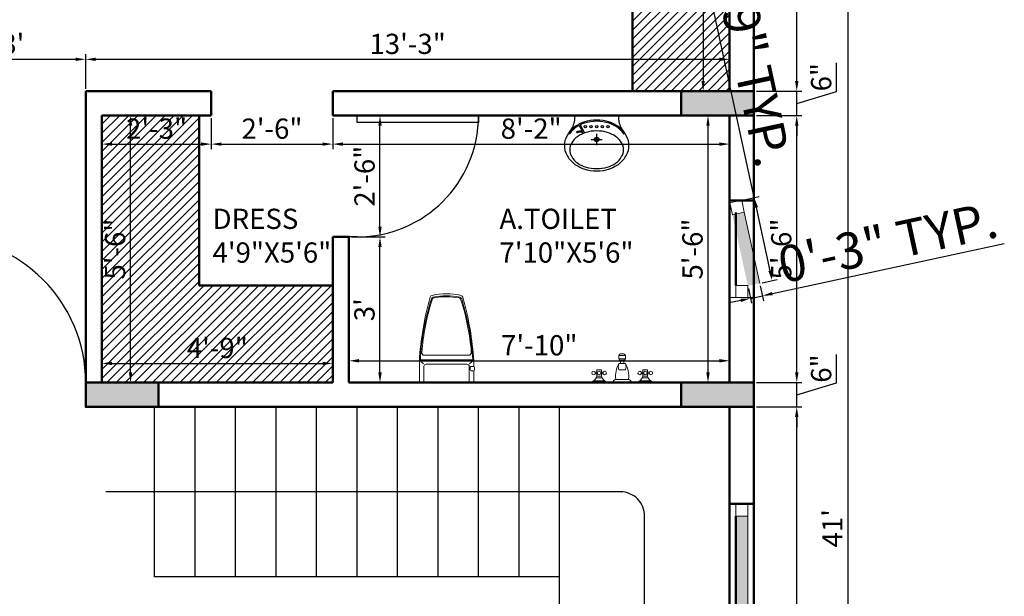
# Model space of a CAD drawing. Units: inches. Extents: x 3064 to 19385, y 846 to 15425.
# Tile 102 of 108: x 7687 to 7930, y 1134 to 1276. Entities that reach past the tile are written whole.
import ezdxf

# ---------------------------------------------------------------- set-up
doc = ezdxf.new("R2010")
doc.units = ezdxf.units.IN
for name, color, linetype, lineweight in [('A-ANNO-DIMS', 2, 'Continuous', 18), ('A-AREA-IDEN', 3, 'Continuous', 18), ('A-COLS', 1, 'Continuous', 35), ('A-DOOR', 3, 'Continuous', 25), ('A-FLOR-FIXT', 9, 'Continuous', 18), ('A-FLOR-STRS', 2, 'Continuous', 25), ('A-FURN-PATT', 252, 'Continuous', 13), ('A-GLAZ', 4, 'Continuous', 18), ('A-WALL', 7, 'Continuous', 50)]:
    doc.layers.add(name, color=color, linetype=linetype, lineweight=lineweight)
doc.layers.add('THIET-BI', color=21, linetype='Continuous')
doc.styles.get("Standard").update_dxf_attribs({"font": 'arial.ttf'})
doc.dimstyles.new('ISO-25', dxfattribs={"dimtxt": 9, "dimasz": 2.5, "dimexe": 1.25, "dimexo": 0.625, "dimtad": 1, "dimdec": 1, "dimlunit": 3, "dimtxsty": 'Standard', "dimcen": 2.5, "dimadec": 0, "dimazin": 0, "dimtfac": 1, "dimtdec": 1, "dimtmove": 0, "dimatfit": 3, "dimfxl": 1, "dimarcsym": 0})
pattern_1 = [(45, (3183.7531, 0), (-1.122532, 1.122532), [])]

# ---------------------------------------------------------------- blocks, each defined once
blk = doc.blocks.new('*U3')
for p, q in [((0, 0), (0, -6)), ((36, 0), (36, -6))]:
    blk.add_line(p, q)
blk.add_lwpolyline([(0, 0), (0, 36), (1.75, 36), (1.75, 0)], close=True)
blk.add_arc((0, 0), 36, 0, 90)
blk = doc.blocks.new('*U4')
for p, q in [((0, 0), (0, -6)), ((30, 0), (30, -6))]:
    blk.add_line(p, q)
blk.add_lwpolyline([(0, 0), (0, 30), (1.75, 30), (1.75, 0)], close=True)
blk.add_arc((0, 0), 30, 0, 90)
blk = doc.blocks.new('*D329')
at = {"layer": 'A-ANNO-DIMS', "color": 0, "lineweight": -2, "transparency": 16777216}
for p, q in [((7868.87, 1180.34), (7880.08, 1180.34)), ((7878.83, 984.84), (7878.83, 1177.84)), ((7862.87, 982.34), (7880.08, 982.34))]:
    blk.add_line(p, q, dxfattribs=at)
at = {"layer": 'A-ANNO-DIMS', "color": 0, "transparency": 16777216}
for points in [[(7878.41, 1177.84), (7879.25, 1177.84), (7878.83, 1180.34)], [(7878.41, 984.84), (7879.25, 984.84), (7878.83, 982.34)]]:
    blk.add_solid(points, dxfattribs=at)
at = {"layer": 'Defpoints', "color": 0, "transparency": 16777216}
for p in [(7868.25, 1180.34), (7878.83, 1180.34), (7862.25, 982.34)]:
    blk.add_point(p, dxfattribs=at)
at = {"layer": 'A-ANNO-DIMS', "color": 0, "transparency": 16777216, "insert": (7875.65, 1081.34), "char_height": 5, "attachment_point": 5, "rotation": 90}
blk.add_mtext('16\'-6"', dxfattribs=at)
blk = doc.blocks.new('*D330')
at = {"layer": 'A-ANNO-DIMS', "color": 0, "lineweight": -2, "transparency": 16777216}
for p, q in [((7878.83, 1188.84), (7878.83, 1191.34)), ((7888.67, 1186.29), (7888.67, 1193.32)), ((7868.87, 1186.34), (7880.08, 1186.34)), ((7878.83, 1180.34), (7878.83, 1186.34)), ((7878.83, 1180.34), (7878.83, 1186.34)), ((7878.83, 1183.34), (7888.67, 1186.29)), ((7868.87, 1180.34), (7880.08, 1180.34)), ((7878.83, 1177.84), (7878.83, 1175.34))]:
    blk.add_line(p, q, dxfattribs=at)
at = {"layer": 'A-ANNO-DIMS', "color": 0, "transparency": 16777216}
for points in [[(7878.41, 1188.84), (7879.25, 1188.84), (7878.83, 1186.34)], [(7878.41, 1177.84), (7879.25, 1177.84), (7878.83, 1180.34)]]:
    blk.add_solid(points, dxfattribs=at)
at = {"layer": 'Defpoints', "color": 0, "transparency": 16777216}
for p in [(7868.25, 1186.34), (7878.83, 1186.34), (7868.25, 1180.34)]:
    blk.add_point(p, dxfattribs=at)
at = {"layer": 'A-ANNO-DIMS', "color": 0, "transparency": 16777216, "insert": (7885.5, 1189.81), "char_height": 5, "attachment_point": 5, "rotation": 90}
blk.add_mtext('6"', dxfattribs=at)
blk = doc.blocks.new('*D331')
at = {"layer": 'A-ANNO-DIMS', "color": 0, "lineweight": -2, "transparency": 16777216}
for p, q in [((7868.87, 1252.34), (7880.08, 1252.34)), ((7878.83, 1188.84), (7878.83, 1249.84)), ((7868.87, 1186.34), (7880.08, 1186.34))]:
    blk.add_line(p, q, dxfattribs=at)
at = {"layer": 'A-ANNO-DIMS', "color": 0, "transparency": 16777216}
for points in [[(7878.41, 1249.84), (7879.25, 1249.84), (7878.83, 1252.34)], [(7878.41, 1188.84), (7879.25, 1188.84), (7878.83, 1186.34)]]:
    blk.add_solid(points, dxfattribs=at)
at = {"layer": 'Defpoints', "color": 0, "transparency": 16777216}
for p in [(7868.25, 1252.34), (7878.83, 1252.34), (7868.25, 1186.34)]:
    blk.add_point(p, dxfattribs=at)
at = {"layer": 'A-ANNO-DIMS', "color": 0, "transparency": 16777216, "insert": (7875.65, 1219.34), "char_height": 5, "attachment_point": 5, "rotation": 90}
blk.add_mtext('5\'-6"', dxfattribs=at)
blk = doc.blocks.new('*D332')
at = {"layer": 'A-ANNO-DIMS', "color": 0, "lineweight": -2, "transparency": 16777216}
for p, q in [((7888.67, 1258.29), (7888.67, 1265.32)), ((7878.83, 1260.84), (7878.83, 1263.34)), ((7868.87, 1258.34), (7880.08, 1258.34)), ((7878.83, 1252.34), (7878.83, 1258.34)), ((7878.83, 1252.34), (7878.83, 1258.34)), ((7878.83, 1255.34), (7888.67, 1258.29)), ((7868.87, 1252.34), (7880.08, 1252.34)), ((7878.83, 1249.84), (7878.83, 1247.34))]:
    blk.add_line(p, q, dxfattribs=at)
at = {"layer": 'A-ANNO-DIMS', "color": 0, "transparency": 16777216}
for points in [[(7878.41, 1260.84), (7879.25, 1260.84), (7878.83, 1258.34)], [(7878.41, 1249.84), (7879.25, 1249.84), (7878.83, 1252.34)]]:
    blk.add_solid(points, dxfattribs=at)
at = {"layer": 'Defpoints', "color": 0, "transparency": 16777216}
for p in [(7868.25, 1258.34), (7878.83, 1258.34), (7868.25, 1252.34)]:
    blk.add_point(p, dxfattribs=at)
at = {"layer": 'A-ANNO-DIMS', "color": 0, "transparency": 16777216, "insert": (7885.5, 1261.81), "char_height": 5, "attachment_point": 5, "rotation": 90}
blk.add_mtext('6"', dxfattribs=at)
blk = doc.blocks.new('*D333')
at = {"layer": 'A-ANNO-DIMS', "color": 0, "lineweight": -2, "transparency": 16777216}
for p, q in [((7862.87, 1390.34), (7880.08, 1390.34)), ((7878.83, 1260.84), (7878.83, 1387.84)), ((7868.87, 1258.34), (7880.08, 1258.34))]:
    blk.add_line(p, q, dxfattribs=at)
at = {"layer": 'A-ANNO-DIMS', "color": 0, "transparency": 16777216}
for points in [[(7878.41, 1387.84), (7879.25, 1387.84), (7878.83, 1390.34)], [(7878.41, 1260.84), (7879.25, 1260.84), (7878.83, 1258.34)]]:
    blk.add_solid(points, dxfattribs=at)
at = {"layer": 'Defpoints', "color": 0, "transparency": 16777216}
for p in [(7862.25, 1390.34), (7878.83, 1390.34), (7868.25, 1258.34)]:
    blk.add_point(p, dxfattribs=at)
at = {"layer": 'A-ANNO-DIMS', "color": 0, "transparency": 16777216, "insert": (7875.69, 1324.34), "char_height": 5, "attachment_point": 5, "rotation": 90}
blk.add_mtext("11'", dxfattribs=at)
blk = doc.blocks.new('*D335')
at = {"layer": 'A-ANNO-DIMS', "color": 0, "lineweight": -2, "transparency": 16777216}
for p, q in [((7868.87, 1396.34), (7892.65, 1396.34)), ((7891.4, 1393.84), (7891.4, 906.84)), ((7868.87, 904.34), (7892.65, 904.34))]:
    blk.add_line(p, q, dxfattribs=at)
at = {"layer": 'A-ANNO-DIMS', "color": 0, "transparency": 16777216}
for points in [[(7890.98, 1393.84), (7891.82, 1393.84), (7891.4, 1396.34)], [(7890.98, 906.84), (7891.82, 906.84), (7891.4, 904.34)]]:
    blk.add_solid(points, dxfattribs=at)
at = {"layer": 'Defpoints', "color": 0, "transparency": 16777216}
for p in [(7868.25, 1396.34), (7868.25, 904.34), (7891.4, 904.34)]:
    blk.add_point(p, dxfattribs=at)
at = {"layer": 'A-ANNO-DIMS', "color": 0, "transparency": 16777216, "insert": (7888.27, 1150.34), "char_height": 5, "attachment_point": 5, "rotation": 90}
blk.add_mtext("41'", dxfattribs=at)
blk = doc.blocks.new('*D230')
at = {"layer": 'A-ANNO-DIMS', "color": 0, "lineweight": -2, "transparency": 16777216}
for p, q in [((7707.87, 1252.34), (7715.58, 1252.34)), ((7714.33, 1188.84), (7714.33, 1249.84)), ((7707.87, 1186.34), (7715.58, 1186.34))]:
    blk.add_line(p, q, dxfattribs=at)
at = {"layer": 'A-ANNO-DIMS', "color": 0, "transparency": 16777216}
for points in [[(7713.91, 1249.84), (7714.74, 1249.84), (7714.33, 1252.34)], [(7713.91, 1188.84), (7714.74, 1188.84), (7714.33, 1186.34)]]:
    blk.add_solid(points, dxfattribs=at)
at = {"layer": 'Defpoints', "color": 0, "transparency": 16777216}
for p in [(7707.25, 1252.34), (7714.33, 1252.34), (7707.25, 1186.34)]:
    blk.add_point(p, dxfattribs=at)
at = {"layer": 'A-ANNO-DIMS', "color": 0, "transparency": 16777216, "insert": (7711.15, 1219.34), "char_height": 5, "attachment_point": 5, "rotation": 90}
blk.add_mtext('5\'-6"', dxfattribs=at)
blk = doc.blocks.new('*D231')
at = {"layer": 'A-ANNO-DIMS', "color": 0, "lineweight": -2, "transparency": 16777216}
for p, q in [((7707.25, 1186.96), (7707.25, 1192.33)), ((7764.25, 1186.96), (7764.25, 1192.33)), ((7709.75, 1191.08), (7761.75, 1191.08))]:
    blk.add_line(p, q, dxfattribs=at)
at = {"layer": 'A-ANNO-DIMS', "color": 0, "transparency": 16777216}
for points in [[(7709.75, 1191.49), (7709.75, 1190.66), (7707.25, 1191.08)], [(7761.75, 1191.49), (7761.75, 1190.66), (7764.25, 1191.08)]]:
    blk.add_solid(points, dxfattribs=at)
at = {"layer": 'Defpoints', "color": 0, "transparency": 16777216}
for p in [(7764.25, 1191.08), (7707.25, 1186.34), (7764.25, 1186.34)]:
    blk.add_point(p, dxfattribs=at)
at = {"layer": 'A-ANNO-DIMS', "color": 0, "transparency": 16777216, "insert": (7735.75, 1194.25), "char_height": 5, "attachment_point": 5}
blk.add_mtext('4\'-9"', dxfattribs=at)
blk = doc.blocks.new('*D250')
at = {"layer": 'A-ANNO-DIMS', "color": 0, "lineweight": -2, "transparency": 16777216}
for p, q in [((7768.25, 1186.96), (7768.25, 1192.98)), ((7770.75, 1191.73), (7859.75, 1191.73)), ((7862.25, 1186.96), (7862.25, 1192.98))]:
    blk.add_line(p, q, dxfattribs=at)
at = {"layer": 'A-ANNO-DIMS', "color": 0, "transparency": 16777216}
for points in [[(7770.75, 1192.15), (7770.75, 1191.31), (7768.25, 1191.73)], [(7859.75, 1192.15), (7859.75, 1191.31), (7862.25, 1191.73)]]:
    blk.add_solid(points, dxfattribs=at)
at = {"layer": 'Defpoints', "color": 0, "transparency": 16777216}
for p in [(7862.25, 1191.73), (7768.25, 1186.34), (7862.25, 1186.34)]:
    blk.add_point(p, dxfattribs=at)
at = {"layer": 'A-ANNO-DIMS', "color": 0, "transparency": 16777216, "insert": (7815.25, 1194.91), "char_height": 5, "attachment_point": 5}
blk.add_mtext('7\'-10"', dxfattribs=at)
blk = doc.blocks.new('*D251')
at = {"layer": 'A-ANNO-DIMS', "color": 0, "lineweight": -2, "transparency": 16777216}
for p, q in [((7861.62, 1252.34), (7855.66, 1252.34)), ((7856.91, 1249.84), (7856.91, 1188.84)), ((7861.62, 1186.34), (7855.66, 1186.34))]:
    blk.add_line(p, q, dxfattribs=at)
at = {"layer": 'A-ANNO-DIMS', "color": 0, "transparency": 16777216}
for points in [[(7856.5, 1249.84), (7857.33, 1249.84), (7856.91, 1252.34)], [(7856.5, 1188.84), (7857.33, 1188.84), (7856.91, 1186.34)]]:
    blk.add_solid(points, dxfattribs=at)
at = {"layer": 'Defpoints', "color": 0, "transparency": 16777216}
for p in [(7862.25, 1252.34), (7856.91, 1186.34), (7862.25, 1186.34)]:
    blk.add_point(p, dxfattribs=at)
at = {"layer": 'A-ANNO-DIMS', "color": 0, "transparency": 16777216, "insert": (7853.73, 1219.34), "char_height": 5, "attachment_point": 5, "rotation": 90}
blk.add_mtext('5\'-6"', dxfattribs=at)
blk = doc.blocks.new('*D252')
at = {"layer": 'A-ANNO-DIMS', "color": 0, "lineweight": -2, "transparency": 16777216}
for p, q in [((7768.87, 1222.34), (7777.17, 1222.34)), ((7775.92, 1188.84), (7775.92, 1219.84)), ((7768.87, 1186.34), (7777.17, 1186.34))]:
    blk.add_line(p, q, dxfattribs=at)
at = {"layer": 'A-ANNO-DIMS', "color": 0, "transparency": 16777216}
for points in [[(7775.51, 1219.84), (7776.34, 1219.84), (7775.92, 1222.34)], [(7775.51, 1188.84), (7776.34, 1188.84), (7775.92, 1186.34)]]:
    blk.add_solid(points, dxfattribs=at)
at = {"layer": 'Defpoints', "color": 0, "transparency": 16777216}
for p in [(7768.25, 1222.34), (7775.92, 1222.34), (7768.25, 1186.34)]:
    blk.add_point(p, dxfattribs=at)
at = {"layer": 'A-ANNO-DIMS', "color": 0, "transparency": 16777216, "insert": (7772.74, 1204.34), "char_height": 5, "attachment_point": 5, "rotation": 90}
blk.add_mtext("3'", dxfattribs=at)
blk = doc.blocks.new('*D253')
at = {"layer": 'A-ANNO-DIMS', "color": 0, "lineweight": -2, "transparency": 16777216}
for p, q in [((7776.55, 1252.34), (7777.17, 1252.34)), ((7775.92, 1224.84), (7775.92, 1249.84)), ((7768.87, 1222.34), (7777.17, 1222.34))]:
    blk.add_line(p, q, dxfattribs=at)
at = {"layer": 'A-ANNO-DIMS', "color": 0, "transparency": 16777216}
for points in [[(7775.51, 1249.84), (7776.34, 1249.84), (7775.92, 1252.34)], [(7775.51, 1224.84), (7776.34, 1224.84), (7775.92, 1222.34)]]:
    blk.add_solid(points, dxfattribs=at)
at = {"layer": 'Defpoints', "color": 0, "transparency": 16777216}
for p in [(7775.92, 1252.34), (7775.92, 1252.34), (7768.25, 1222.34)]:
    blk.add_point(p, dxfattribs=at)
at = {"layer": 'A-ANNO-DIMS', "color": 0, "transparency": 16777216, "insert": (7772.75, 1237.34), "char_height": 5, "attachment_point": 5, "rotation": 90}
blk.add_mtext('2\'-6"', dxfattribs=at)
blk = doc.blocks.new('*D254')
at = {"layer": 'A-ANNO-DIMS', "color": 0, "lineweight": -2, "transparency": 16777216}
for p, q in [((7707.25, 1251.71), (7707.25, 1244.02)), ((7734.25, 1251.71), (7734.25, 1244.02)), ((7709.75, 1245.27), (7731.75, 1245.27))]:
    blk.add_line(p, q, dxfattribs=at)
at = {"layer": 'A-ANNO-DIMS', "color": 0, "transparency": 16777216}
for points in [[(7709.75, 1245.69), (7709.75, 1244.86), (7707.25, 1245.27)], [(7731.75, 1245.69), (7731.75, 1244.86), (7734.25, 1245.27)]]:
    blk.add_solid(points, dxfattribs=at)
at = {"layer": 'Defpoints', "color": 0, "transparency": 16777216}
for p in [(7707.25, 1252.34), (7734.25, 1252.34), (7734.25, 1245.27)]:
    blk.add_point(p, dxfattribs=at)
at = {"layer": 'A-ANNO-DIMS', "color": 0, "transparency": 16777216, "insert": (7720.75, 1248.45), "char_height": 5, "attachment_point": 5}
blk.add_mtext('2\'-3"', dxfattribs=at)
blk = doc.blocks.new('*D246')
at = {"layer": 'A-ANNO-DIMS', "color": 0, "lineweight": -2, "transparency": 16777216}
for p, q in [((7734.25, 1251.71), (7734.25, 1244.02)), ((7764.25, 1251.71), (7764.25, 1244.02)), ((7736.75, 1245.27), (7761.75, 1245.27))]:
    blk.add_line(p, q, dxfattribs=at)
at = {"layer": 'A-ANNO-DIMS', "color": 0, "transparency": 16777216}
for points in [[(7736.75, 1245.69), (7736.75, 1244.86), (7734.25, 1245.27)], [(7761.75, 1245.69), (7761.75, 1244.86), (7764.25, 1245.27)]]:
    blk.add_solid(points, dxfattribs=at)
at = {"layer": 'Defpoints', "color": 0, "transparency": 16777216}
for p in [(7734.25, 1252.34), (7764.25, 1252.34), (7764.25, 1245.27)]:
    blk.add_point(p, dxfattribs=at)
at = {"layer": 'A-ANNO-DIMS', "color": 0, "transparency": 16777216, "insert": (7749.25, 1248.45), "char_height": 5, "attachment_point": 5}
blk.add_mtext('2\'-6"', dxfattribs=at)
blk = doc.blocks.new('*D247')
at = {"layer": 'A-ANNO-DIMS', "color": 0, "lineweight": -2, "transparency": 16777216}
for p, q in [((7764.25, 1251.71), (7764.25, 1244.02)), ((7862.25, 1251.71), (7862.25, 1244.02)), ((7766.75, 1245.27), (7859.75, 1245.27))]:
    blk.add_line(p, q, dxfattribs=at)
at = {"layer": 'A-ANNO-DIMS', "color": 0, "transparency": 16777216}
for points in [[(7766.75, 1245.69), (7766.75, 1244.86), (7764.25, 1245.27)], [(7859.75, 1245.69), (7859.75, 1244.86), (7862.25, 1245.27)]]:
    blk.add_solid(points, dxfattribs=at)
at = {"layer": 'Defpoints', "color": 0, "transparency": 16777216}
for p in [(7764.25, 1252.34), (7862.25, 1252.34), (7862.25, 1245.27)]:
    blk.add_point(p, dxfattribs=at)
at = {"layer": 'A-ANNO-DIMS', "color": 0, "transparency": 16777216, "insert": (7813.25, 1248.45), "char_height": 5, "attachment_point": 5}
blk.add_mtext('8\'-2"', dxfattribs=at)
blk = doc.blocks.new('*D249')
at = {"layer": 'A-ANNO-DIMS', "color": 0, "lineweight": -2, "transparency": 16777216}
for p, q in [((7861.62, 1390.34), (7854.47, 1390.34)), ((7855.72, 1387.84), (7855.72, 1260.84)), ((7861.62, 1258.34), (7854.47, 1258.34))]:
    blk.add_line(p, q, dxfattribs=at)
at = {"layer": 'A-ANNO-DIMS', "color": 0, "transparency": 16777216}
for points in [[(7855.3, 1387.84), (7856.13, 1387.84), (7855.72, 1390.34)], [(7855.3, 1260.84), (7856.13, 1260.84), (7855.72, 1258.34)]]:
    blk.add_solid(points, dxfattribs=at)
at = {"layer": 'Defpoints', "color": 0, "transparency": 16777216}
for p in [(7862.25, 1390.34), (7855.72, 1258.34), (7862.25, 1258.34)]:
    blk.add_point(p, dxfattribs=at)
at = {"layer": 'A-ANNO-DIMS', "color": 0, "transparency": 16777216, "insert": (7852.58, 1324.34), "char_height": 5, "attachment_point": 5, "rotation": 90}
blk.add_mtext("11'", dxfattribs=at)
blk = doc.blocks.new('*D242')
at = {"layer": 'A-ANNO-DIMS', "color": 0, "lineweight": -2, "transparency": 16777216}
for p, q in [((7703.25, 1258.96), (7703.25, 1267.47)), ((7862.25, 1258.96), (7862.25, 1267.47)), ((7859.75, 1266.22), (7705.75, 1266.22))]:
    blk.add_line(p, q, dxfattribs=at)
at = {"layer": 'A-ANNO-DIMS', "color": 0, "transparency": 16777216}
for points in [[(7705.75, 1266.64), (7705.75, 1265.81), (7703.25, 1266.22)], [(7859.75, 1266.64), (7859.75, 1265.81), (7862.25, 1266.22)]]:
    blk.add_solid(points, dxfattribs=at)
at = {"layer": 'Defpoints', "color": 0, "transparency": 16777216}
for p in [(7703.25, 1266.22), (7703.25, 1258.34), (7862.25, 1258.34)]:
    blk.add_point(p, dxfattribs=at)
at = {"layer": 'A-ANNO-DIMS', "color": 0, "transparency": 16777216, "insert": (7782.75, 1269.4), "char_height": 5, "attachment_point": 5}
blk.add_mtext('13\'-3"', dxfattribs=at)
blk = doc.blocks.new('*D243')
at = {"layer": 'A-ANNO-DIMS', "color": 0, "lineweight": -2, "transparency": 16777216}
for p, q in [((7667.25, 1269.71), (7667.25, 1264.97)), ((7703.25, 1258.96), (7703.25, 1267.47)), ((7700.75, 1266.22), (7669.75, 1266.22))]:
    blk.add_line(p, q, dxfattribs=at)
at = {"layer": 'A-ANNO-DIMS', "color": 0, "transparency": 16777216}
for points in [[(7669.75, 1266.64), (7669.75, 1265.81), (7667.25, 1266.22)], [(7700.75, 1266.64), (7700.75, 1265.81), (7703.25, 1266.22)]]:
    blk.add_solid(points, dxfattribs=at)
at = {"layer": 'Defpoints', "color": 0, "transparency": 16777216}
for p in [(7667.25, 1270.34), (7667.25, 1266.22), (7703.25, 1258.34)]:
    blk.add_point(p, dxfattribs=at)
at = {"layer": 'A-ANNO-DIMS', "color": 0, "transparency": 16777216, "insert": (7685.25, 1269.4), "char_height": 5, "attachment_point": 5}
blk.add_mtext("3'", dxfattribs=at)
blk = doc.blocks.new('A$C430D11A0')
at = {"layer": 'THIET-BI'}
for p, q in [((90, 445), (90, 485)), ((475, 485), (90, 485)), ((475, 483), (90, 483)), ((475, 445), (475, 485)), ((129.4, 398.5), (158.2, 344.4)), ((138.3, 403), (176, 332.4)), ((233.4, 275.5), (331.9, 275.5)), ((282.5, 226.2), (282.5, 324.8))]:
    blk.add_line(p, q, dxfattribs=at)
for points in [[(565, 222.5, 0.121635), (544.7, 304.8, 0.10526), (482.3, 379.8, 0.088175), (393.4, 427.4, 0.079002), (282.5, 445, 0.079002), (171.6, 427.4, 0.088175), (82.7, 379.8, 0.10526), (20.3, 304.8, 0.121635), (0, 222.5, 0.121635), (20.3, 140.2, 0.10526), (82.7, 65.2, 0.088175), (171.6, 17.6, 0.079002), (282.5, 0, 0.079002), (393.4, 17.6, 0.088175), (482.3, 65.2, 0.10526), (544.7, 140.2, 0.121635)], [(517.5, 185, 0.134042), (501.2, 244.9, 0.106817), (448.7, 301.7, 0.082468), (375.6, 336.7, 0.070874), (282.5, 350, 0.070874), (189.4, 336.7, 0.082468), (116.3, 301.7, 0.106817), (63.8, 244.9, 0.134042), (47.5, 185, 0.134042), (63.8, 125.1, 0.106817), (116.3, 68.3, 0.082468), (189.4, 33.3, 0.070874), (282.5, 20, 0.070874), (375.6, 33.3, 0.082468), (448.7, 68.3, 0.106817), (501.2, 125.1, 0.134042)]]:
    blk.add_lwpolyline(points, format="xyb", close=True, dxfattribs=at)
for points in [[(522.9, 321.6, 0.07708), (476.1, 372, 0.088175), (390.3, 417.9, 0.079002), (282.5, 435, 0.079002), (174.7, 417.9, 0.035427), (138.3, 403, 0.07708)], [(129.4, 398.5, 0.043566), (88.9, 372, 0.07708), (42.1, 321.6, 0.041486)]]:
    blk.add_lwpolyline(points, format="xyb", dxfattribs=at)
for centre, radius in [((182.5, 388.2), 10.5), ((232.5, 388.2), 10.5), ((282.5, 388.2), 10.5), ((332.5, 388.2), 10.5), ((382.5, 388.2), 10.5), ((282.5, 275.5), 20), ((282.5, 275.5), 15)]:
    blk.add_circle(centre, radius, dxfattribs=at)
for centre, radius, start, end in [((-103.8, 468.9), 195.3, 320.8253, 352.95569), ((668.8, 468.9), 195.3, 187.04431, 219.1747), ((136.4, 285.4), 62.9, 69.64296, 123.47738), ((136.4, 285.4), 52.9, 55.24551, 123.47738)]:
    blk.add_arc(centre, radius, start, end, dxfattribs=at)
blk = doc.blocks.new('WC-P05')
for p, q in [((-202.4, 531.6), (-202.4, 439.1)), ((-192.4, 541.6), (262.6, 541.6)), ((-163.4, 541.6), (-163.4, 400.6)), ((233.6, 541.6), (233.6, 400.6)), ((272.6, 531.6), (272.6, 351.6)), ((-201.4, 439.1), (-180.4, 439.1)), ((-210.4, 430.1), (-210.4, 409.1)), ((-202.4, 400.1), (-202.4, 351.6)), ((-201.4, 400.1), (-180.4, 400.1)), ((-166.9, 378.6), (-188.2, 357.3)), ((-171.4, 430.1), (-171.4, 409.1)), ((-143.4, 380.6), (213.6, 380.6)), ((237.1, 378.6), (258.4, 357.3)), ((-192.4, 341.6), (262.6, 341.6)), ((-159.3, 302.6), (229.5, 302.6))]:
    blk.add_line(p, q)
blk.add_lwpolyline([(-90.9, -221.9, 0.114547), (161, -222, 0.114547)], format="xyb")
for centre, radius, start, end in [((-192.4, 531.6), 10, 90, 180), ((262.6, 531.6), 10, 0, 90), ((-201.4, 430.1), 9, 90, 180), ((-180.4, 430.1), 9, 0, 90), ((-201.4, 409.1), 9, 180, 270), ((2308.9, 492.3), 2515.2, 183.20675, 196.12415), ((-192.4, 351.6), 10, 180, 270), ((-180.4, 409.1), 9, 270, 0), ((-143.4, 400.6), 20, 180, 270), ((-2238.7, 492.3), 2515.2, 343.87268, 356.79325), ((213.6, 400.6), 20, 270, 0), ((262.6, 351.6), 10, 270, 0), ((1906, 447.2), 2102.6, 182.87428, 197.65536), ((-159.3, 280.1), 22.5, 90, 184.62462), ((1905.9, 447.2), 2094.5, 184.62454, 197.52765), ((-1835.8, 447.2), 2094.6, 342.46396, 355.37538), ((-1835.8, 447.2), 2102.6, 342.34464, 357.12572), ((229.5, 280.1), 22.5, 355.37538, 90), ((-85.8, -199.9), 22.5, 196.12415, 256.89941), ((-76.1, -183.7), 22.5, 197.65536, 257.50587), ((-69.9, -176.8), 22.5, 197.52765, 258.10049), ((35.1, 318), 536.4, 257.50587, 282.49413), ((35.7, 324.3), 534.7, 258.10049, 281.73735), ((139.9, -177.1), 22.5, 281.73735, 342.46396), ((146.2, -183.7), 22.5, 282.49413, 342.34464), ((155.9, -200.1), 22.5, 283.03778, 343.87268)]:
    blk.add_arc(centre, radius, start, end)
blk = doc.blocks.new('Faucet - Bathroom front')
for p, q in [((-0.5, 4.25), (0.5, 4.25)), ((0.5, 3.75), (-0.5, 3.75)), ((-0.25, 3), (-0.25, 3.5)), ((0.25, 3.5), (0.25, 3)), ((-4, 1.625), (-4.25, 1.625)), ((-3.25, 1.625), (-3, 1.625)), ((-0.5, 3), (0.5, 3)), ((0.5, 2), (-0.5, 2)), ((3.25, 1.625), (3, 1.625)), ((4, 1.625), (4.25, 1.625)), ((-5, 0), (-2.25, 0)), ((-4.5087, 0.25), (-2.7408, 0.25)), ((-4, 1.375), (-4.25, 1.375)), ((-3.1442, 0.75), (-4.0979, 0.75)), ((-3.25, 1.375), (-3, 1.375)), ((-1.5, 0), (1.5, 0)), ((-1, 0.5), (1, 0.5)), ((2.25, 0), (5, 0)), ((2.7413, 0.25), (4.5092, 0.25)), ((3.25, 1.375), (3, 1.375)), ((4.1058, 0.75), (3.1521, 0.75)), ((4, 1.375), (4.25, 1.375))]:
    blk.add_line(p, q)
for points in [[(-0.5, 3.75), (-0.5, 4.25)], [(-0.25, 4.5), (0.25, 4.5)], [(0.25, 3.5), (-0.25, 3.5)], [(0.5, 4.25), (0.5, 3.75)]]:
    blk.add_lwpolyline(points)
for points in [[(-4, 1), (-4, 2), (-3.25, 2), (-3.25, 1)], [(3.25, 1), (3.25, 2), (4, 2), (4, 1)]]:
    blk.add_lwpolyline(points, close=True)
for centre in [(-4.5, 1.5), (-3.625, 1.5), (-2.75, 1.5), (2.75, 1.5), (3.625, 1.5), (4.5, 1.5)]:
    blk.add_circle(centre, 0.2795)
for centre, radius, start, end in [((-0.2575, 4.2575), 0.2426, 88.22243, 181.7776), ((-0.2575, 3.7425), 0.2426, 178.2224, 271.7776), ((0.2575, 4.2575), 0.2426, 358.2224, 91.77757), ((0.2575, 3.7425), 0.2426, 268.2224, 1.777565), ((3, 1), 4.0311, 150.2551, 187.125), ((0.6413, 2.5), 1.246, 156.3417, 203.6583), ((-3, 1), 4.0311, 352.875, 29.74488), ((-0.6413, 2.5), 1.246, 336.3417, 23.65835), ((-5.375, 1.375), 1.4252, 285.2551, 344.7449), ((-1.875, 1.375), 1.4252, 195.2551, 254.7449), ((-0.7962, -0.2038), 0.7327, 106.1502, 163.8498), ((0.7962, -0.2038), 0.7327, 16.1502, 73.84979), ((1.875, 1.375), 1.4252, 285.2551, 344.7449), ((5.375, 1.375), 1.4252, 195.2551, 254.7449)]:
    blk.add_arc(centre, radius, start, end)
blk = doc.blocks.new('WIN-600')
h = blk.add_hatch(color=256)
h.dxf.hatch_style = 1
h.paths.add_polyline_path([(3, 18), (0, 18), (0, 0), (3, 0)])
blk.add_line((3, 18), (3, 0))
blk.add_lwpolyline([(3, 18), (0, 18), (0, 21), (3, 21)], close=True)
blk = doc.blocks.new('WIN-1800-PAIR')
h = blk.add_hatch(color=256)
h.dxf.hatch_style = 1
h.paths.add_polyline_path([(0, 0), (3, 0), (3, 70.5), (0, 70.5)])
h.paths.add_polyline_path([(3, 144), (0, 144), (0, 73.5), (3, 73.5)])
blk.add_line((3, 144), (3, 73.5))
blk.add_lwpolyline([(3, 144), (0, 144), (0, 147), (3, 147)], close=True)
blk = doc.blocks.new('*D439')
at = {"layer": 'A-ANNO-DIMS', "color": 0, "lineweight": -2, "transparency": 16777216}
for p, q in [((7868.32, 1232.06), (7835.74, 1382.55)), ((7865.85, 1231.53), (7869.54, 1232.32)), ((7872.24, 1213.98), (7868.85, 1229.62)), ((7870.3, 1211), (7873.99, 1211.8))]:
    blk.add_line(p, q, dxfattribs=at)
at = {"layer": 'A-ANNO-DIMS', "color": 0, "transparency": 16777216}
for points in [[(7869.26, 1229.7), (7868.44, 1229.53), (7868.32, 1232.06)], [(7872.64, 1214.07), (7871.83, 1213.89), (7872.76, 1211.54)]]:
    blk.add_solid(points, dxfattribs=at)
at = {"layer": 'Defpoints', "color": 0, "transparency": 16777216}
for p in [(7865.24, 1231.39), (7868.32, 1232.06), (7869.69, 1210.87)]:
    blk.add_point(p, dxfattribs=at)
at = {"layer": 'A-ANNO-DIMS', "color": 0, "transparency": 16777216, "insert": (7856.93, 1309.64), "char_height": 9, "attachment_point": 5, "rotation": 282.2157}
blk.add_mtext('WINDOW W600 1\'-9" TYP.', dxfattribs=at)
blk = doc.blocks.new('*D440')
at = {"layer": 'A-ANNO-DIMS', "color": 0, "lineweight": -2, "transparency": 16777216}
for p, q in [((7872.8, 1208.32), (7930.08, 1220.72)), ((7866.89, 1209.62), (7867.68, 1205.93)), ((7869.82, 1210.26), (7870.62, 1206.57)), ((7864.98, 1206.63), (7862.53, 1206.1)), ((7867.42, 1207.16), (7870.35, 1207.79))]:
    blk.add_line(p, q, dxfattribs=at)
at = {"layer": 'A-ANNO-DIMS', "color": 0, "transparency": 16777216}
for points in [[(7872.71, 1208.73), (7872.88, 1207.91), (7870.35, 1207.79)], [(7864.89, 1207.03), (7865.06, 1206.22), (7867.42, 1207.16)]]:
    blk.add_solid(points, dxfattribs=at)
at = {"layer": 'Defpoints', "color": 0, "transparency": 16777216}
for p in [(7869.69, 1210.87), (7866.75, 1210.23), (7870.35, 1207.79)]:
    blk.add_point(p, dxfattribs=at)
at = {"layer": 'A-ANNO-DIMS', "color": 0, "transparency": 16777216, "insert": (7901.55, 1219.89), "char_height": 9, "attachment_point": 5, "rotation": 12.2157}
blk.add_mtext('0\'-3" TYP.', dxfattribs=at)

msp = doc.modelspace()

# ---------------------------------------------------------------- hatches: boundary and pattern name
at = {"layer": 'A-COLS'}
h = msp.add_hatch(color=256, dxfattribs=at)
h.dxf.hatch_style = 1
h.paths.add_polyline_path([(7868.25, 1252.34), (7868.25, 1258.34), (7850.25, 1258.34), (7850.25, 1252.34)])
h = msp.add_hatch(color=256, dxfattribs=at)
h.dxf.hatch_style = 1
h.paths.add_polyline_path([(7721.25, 1180.34), (7721.25, 1186.34), (7703.25, 1186.34), (7703.25, 1180.34)])
h = msp.add_hatch(color=256, dxfattribs=at)
h.dxf.hatch_style = 1
h.paths.add_polyline_path([(7868.25, 1180.34), (7868.25, 1186.34), (7850.25, 1186.34), (7850.25, 1180.34)])
at = {"layer": 'A-FURN-PATT'}
h = msp.add_hatch(dxfattribs=at)
h.set_pattern_fill('ANSI31', color=256, scale=0.5)
h.set_pattern_definition(pattern_1)
h.paths.add_polyline_path([(7838.25, 1258.34), (7862.25, 1258.34), (7862.25, 1390.34), (7838.25, 1390.34)])
h = msp.add_hatch(dxfattribs=at)
h.set_pattern_fill('ANSI31', color=256, scale=0.5)
h.set_pattern_definition(pattern_1)
h.paths.add_polyline_path([(7731.25, 1210.34), (7731.25, 1252.34), (7707.25, 1252.34), (7707.25, 1186.34), (7721.25, 1186.34), (7764.25, 1186.34), (7764.25, 1210.34)])

# ---------------------------------------------------------------- linework, layer by layer
at = {"layer": 'A-FLOR-STRS'}
for p, q in [((7720.25, 1138.34), (7720.25, 1180.34)), ((7730.25, 1138.34), (7730.25, 1180.34)), ((7740.25, 1138.34), (7740.25, 1180.34)), ((7750.25, 1138.34), (7750.25, 1180.34)), ((7760.25, 1138.34), (7760.25, 1180.34)), ((7770.25, 1138.34), (7770.25, 1180.34)), ((7780.25, 1138.34), (7780.25, 1180.34)), ((7790.25, 1138.34), (7790.25, 1180.34)), ((7800.25, 1138.34), (7800.25, 1180.34)), ((7810.25, 1138.34), (7810.25, 1180.34)), ((7820.25, 1024.34), (7820.25, 1180.34)), ((7820.25, 1138.34), (7720.25, 1138.34))]:
    msp.add_line(p, q, dxfattribs=at)
msp.add_lwpolyline([(7727.74, 1003.34), (7835.25, 1003.34, 0.414214), (7841.25, 1009.34), (7841.25, 1153.34, 0.414214), (7835.25, 1159.34), (7708.25, 1159.34)], format="xyb", dxfattribs=at)
at = {"layer": 'A-GLAZ'}
msp.add_line((7862.25, 1207.34), (7868.25, 1207.34), dxfattribs=at)
msp.add_lwpolyline([(7866.75, 1207.34), (7863.75, 1207.34), (7863.75, 1210.34), (7866.75, 1210.34)], close=True, dxfattribs=at)
at = {"layer": 'A-WALL'}
for p, q in [((7868.25, 904.34), (7868.25, 1396.34)), ((7838.25, 1258.34), (7838.25, 1390.34)), ((7862.25, 1258.34), (7862.25, 1390.34)), ((7734.25, 1258.34), (7703.25, 1258.34)), ((7703.25, 1258.34), (7703.25, 1180.34)), ((7734.25, 1258.34), (7734.25, 1252.34)), ((7862.25, 1258.34), (7764.25, 1258.34)), ((7764.25, 1258.34), (7764.25, 1252.34)), ((7734.25, 1252.34), (7707.25, 1252.34)), ((7707.25, 1252.34), (7707.25, 1186.34)), ((7731.25, 1252.34), (7731.25, 1210.34)), ((7862.25, 1252.34), (7764.25, 1252.34)), ((7862.25, 1186.34), (7862.25, 1252.34)), ((7862.25, 1231.34), (7868.25, 1231.34)), ((7863.75, 1228.34), (7863.75, 1210.34)), ((7768.25, 1222.34), (7764.25, 1222.34)), ((7764.25, 1222.34), (7764.25, 1186.34)), ((7768.25, 1186.34), (7768.25, 1222.34)), ((7764.25, 1210.34), (7731.25, 1210.34)), ((7764.25, 1186.34), (7707.25, 1186.34)), ((7862.25, 1186.34), (7768.25, 1186.34)), ((7862.25, 1180.34), (7703.25, 1180.34)), ((7862.25, 982.34), (7862.25, 1180.34)), ((7868.25, 1156.34), (7862.25, 1156.34)), ((7863.75, 1153.34), (7863.75, 1082.84))]:
    msp.add_line(p, q, dxfattribs=at)
for points in [[(7868.25, 1258.34), (7850.25, 1258.34), (7850.25, 1252.34), (7868.25, 1252.34)], [(7721.25, 1186.34), (7703.25, 1186.34), (7703.25, 1180.34), (7721.25, 1180.34)], [(7868.25, 1186.34), (7850.25, 1186.34), (7850.25, 1180.34), (7868.25, 1180.34)]]:
    msp.add_lwpolyline(points, close=True, dxfattribs=at)

# ---------------------------------------------------------------- block references
at = {"layer": 'A-DOOR', "rotation": 270}
msp.add_blockref('*U4', (7770.25, 1252.34), dxfattribs=at)
at = {"layer": 'A-DOOR'}
msp.add_blockref('*U3', (7667.25, 1186.34), dxfattribs=at)
at = {"layer": 'A-FLOR-FIXT'}
for name, p, xscale, yscale, zscale in [('A$C430D11A0', (7821.45, 1238.65), 0.0282220760332506, 0.0282220760332506, 0.0282220760332506), ('Faucet - Bathroom front', (7835.72, 1186.34), 1.573166238287219, 1.573166238287219, 1.573166238287219)]:
    msp.add_blockref(name, p, dxfattribs=dict(at, xscale=xscale, yscale=yscale, zscale=zscale))
at = {"layer": 'A-FLOR-FIXT', "xscale": 0.0282220760332506, "yscale": 0.0282220760332506, "zscale": 0.0282220760332506, "rotation": 180}
msp.add_blockref('WC-P05', (7793.34, 1201.63), dxfattribs=at)
at = {"layer": 'A-GLAZ', "rotation": 12.21571913412712}
msp.add_blockref('WIN-600', (7866.75, 1210.23), dxfattribs=at)
at = {"layer": 'A-GLAZ'}
msp.add_blockref('WIN-1800-PAIR', (7863.75, 1009.34), dxfattribs=at)

# ---------------------------------------------------------------- texts
at = {"layer": 'A-AREA-IDEN', "char_height": 5, "attachment_point": 1}
for s, insert in [('DRESS\\P4\'9"X5\'6"', (7734.58, 1229.31)), ('A.TOILET\\P7\'10"X5\'6"', (7805.42, 1229.31))]:
    msp.add_mtext_dynamic_manual_height_columns(s, width=67.5924, gutter_width=12.5, heights=[0], dxfattribs=dict(at, insert=insert))

# ---------------------------------------------------------------- dimensions: what is measured, and where the dimension line sits
at = {"layer": 'A-ANNO-DIMS'}
for base, p1, p2, override, picture, middle in [((7891.4, 904.34), (7868.25, 1396.34), (7868.25, 904.34), {"dimtxt": 5, "dimclrd": 0, "dimclre": 0, "dimclrt": 0}, '*D335', (7888.27, 1150.34)), ((7855.72, 1258.34), (7862.25, 1390.34), (7862.25, 1258.34), {"dimtxt": 5, "dimclrd": 0, "dimclre": 0, "dimclrt": 0}, '*D249', (7852.58, 1324.34)), ((7878.83, 1390.34), (7868.25, 1258.34), (7862.25, 1390.34), {"dimtxt": 5, "dimclrd": 0, "dimclre": 0, "dimclrt": 0, "dimtmove": 1}, '*D333', (7875.69, 1324.34)), ((7878.83, 1258.34), (7868.25, 1252.34), (7868.25, 1258.34), {"dimtxt": 5, "dimclrd": 0, "dimclre": 0, "dimclrt": 0, "dimtmove": 1}, '*D332', (7885.5, 1258.92)), ((7714.33, 1252.34), (7707.25, 1186.34), (7707.25, 1252.34), {"dimtxt": 5, "dimclrd": 0, "dimclre": 0, "dimclrt": 0}, '*D230', (7711.15, 1219.34)), ((7775.92, 1252.34), (7768.25, 1222.34), (7775.92, 1252.34), {"dimtxt": 5, "dimclrd": 0, "dimclre": 0, "dimclrt": 0, "dimtmove": 1}, '*D253', (7772.75, 1237.34)), ((7856.91, 1186.34), (7862.25, 1252.34), (7862.25, 1186.34), {"dimtxt": 5, "dimclrd": 0, "dimclre": 0, "dimclrt": 0}, '*D251', (7853.73, 1219.34)), ((7878.83, 1252.34), (7868.25, 1186.34), (7868.25, 1252.34), {"dimtxt": 5, "dimclrd": 0, "dimclre": 0, "dimclrt": 0, "dimtmove": 1}, '*D331', (7875.65, 1219.34)), ((7775.92, 1222.34), (7768.25, 1186.34), (7768.25, 1222.34), {"dimtxt": 5, "dimclrd": 0, "dimclre": 0, "dimclrt": 0}, '*D252', (7772.74, 1204.34)), ((7878.83, 1186.34), (7868.25, 1180.34), (7868.25, 1186.34), {"dimtxt": 5, "dimclrd": 0, "dimclre": 0, "dimclrt": 0, "dimtmove": 1}, '*D330', (7885.5, 1186.92)), ((7878.83, 1180.34), (7862.25, 982.34), (7868.25, 1180.34), {"dimtxt": 5, "dimclrd": 0, "dimclre": 0, "dimclrt": 0, "dimtmove": 1}, '*D329', (7875.65, 1081.34))]:
    dim = msp.add_linear_dim(base=base, p1=p1, p2=p2, angle=90, dimstyle='ISO-25', override=override, dxfattribs=at)
    dim.commit()
    dim.dimension.update_dxf_attribs({"geometry": picture, "text_midpoint": middle})
for base, p1, p2, angle, text, picture, middle in [((7868.32, 1232.06), (7869.69, 1210.87), (7865.24, 1231.39), 102.2157, 'WINDOW W600 <> TYP.', '*D439', (7856.93, 1309.64)), ((7870.35, 1207.79), (7866.75, 1210.23), (7869.69, 1210.87), 12.2157, '<> TYP.', '*D440', (7901.55, 1219.89))]:
    dim = msp.add_linear_dim(base=base, p1=p1, p2=p2, angle=angle, text=text, dimstyle='ISO-25', override={"dimdec": 1, "dimrnd": 0, "dimzin": 1, "dimlunit": 4, "dimfrac": 2}, dxfattribs=at)
    dim.commit()
    dim.dimension.update_dxf_attribs({"geometry": picture, "text_midpoint": middle})
for base, p1, p2, override, picture, middle in [((7667.25, 1266.22), (7703.25, 1258.34), (7667.25, 1270.34), {"dimtxt": 5, "dimclrd": 0, "dimclre": 0, "dimclrt": 0, "dimtmove": 1}, '*D243', (7685.25, 1269.4)), ((7703.25, 1266.22), (7862.25, 1258.34), (7703.25, 1258.34), {"dimtxt": 5, "dimclrd": 0, "dimclre": 0, "dimclrt": 0}, '*D242', (7782.75, 1269.4)), ((7734.25, 1245.27), (7707.25, 1252.34), (7734.25, 1252.34), {"dimtxt": 5, "dimclrd": 0, "dimclre": 0, "dimclrt": 0}, '*D254', (7720.75, 1248.45)), ((7764.25, 1245.27), (7734.25, 1252.34), (7764.25, 1252.34), {"dimtxt": 5, "dimclrd": 0, "dimclre": 0, "dimclrt": 0, "dimtmove": 1}, '*D246', (7749.25, 1248.45)), ((7862.25, 1245.27), (7764.25, 1252.34), (7862.25, 1252.34), {"dimtxt": 5, "dimclrd": 0, "dimclre": 0, "dimclrt": 0, "dimtmove": 1}, '*D247', (7813.25, 1248.45)), ((7764.25, 1191.08), (7707.25, 1186.34), (7764.25, 1186.34), {"dimtxt": 5, "dimclrd": 0, "dimclre": 0, "dimclrt": 0}, '*D231', (7735.75, 1194.25)), ((7862.25, 1191.73), (7768.25, 1186.34), (7862.25, 1186.34), {"dimtxt": 5, "dimclrd": 0, "dimclre": 0, "dimclrt": 0}, '*D250', (7815.25, 1194.91))]:
    dim = msp.add_linear_dim(base=base, p1=p1, p2=p2, dimstyle='ISO-25', override=override, dxfattribs=at)
    dim.commit()
    dim.dimension.update_dxf_attribs({"geometry": picture, "text_midpoint": middle})

doc.saveas('drawing.dxf')
